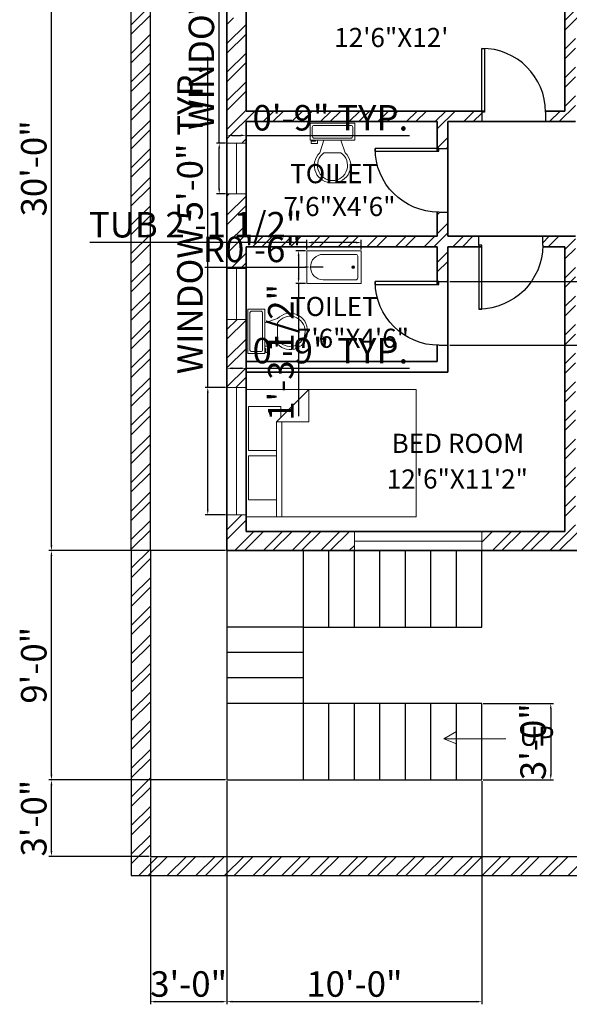
# Model space of a CAD drawing. Units: inches. Extents: x 2588 to 3237, y 2402 to 3178.
# Tile 1 of 4: x 2619 to 2878, y 2412 to 2876. Entities that reach past the tile are written whole.
import ezdxf

# ---------------------------------------------------------------- set-up
doc = ezdxf.new("R2010")
doc.units = ezdxf.units.IN
for name, color, linetype, lineweight in [('A-ANNO-DIMS', 2, 'Continuous', 18), ('A-ANNO-SYMB', 7, 'Continuous', 18), ('A-ANNO-TEXT', 7, 'Continuous', 18), ('A-AREA-IDEN', 7, 'Continuous', 25), ('A-DOOR', 3, 'Continuous', 25), ('A-FLOR-FIXT', 9, 'Continuous', 18), ('A-FLOR-STRS', 7, 'Continuous', 25), ('A-FURN', 8, 'Continuous', 18), ('A-GLAZ', 4, 'Continuous', 18), ('A-WALL-PATT', 252, 'Continuous', 13), ('L-WALL', 7, 'Continuous', 30), ('L-WALL-PATT', 252, 'Continuous', 13), ('wall', 210, 'Continuous', 35)]:
    doc.layers.add(name, color=color, linetype=linetype, lineweight=lineweight)
doc.styles.get("Standard").update_dxf_attribs({"font": 'arial.ttf'})
doc.dimstyles.new('ISO-25', dxfattribs={"dimtxt": 12, "dimasz": 2.5, "dimexe": 1.25, "dimexo": 0.625, "dimtad": 1, "dimdec": 1, "dimlunit": 4, "dimtxsty": 'Standard', "dimcen": 2.5, "dimadec": 0, "dimazin": 0, "dimtfac": 1, "dimtdec": 1, "dimtmove": 0, "dimatfit": 3, "dimfxl": 1, "dimarcsym": 0})

# ---------------------------------------------------------------- blocks, each defined once
blk = doc.blocks.new('Bed - Queen')
for p, q in [((0, -80.00003), (0, 0)), ((0, 0), (59.99999, 0)), ((59.99999, 0), (59.99999, -80.00003)), ((7.99999, -1.2), (28.79998, -1.2)), ((7.99999, -14.4), (7.99999, -1.2)), ((28.79998, -1.2), (28.79998, -14.4)), ((31.19999, -1.2), (51.99999, -1.2)), ((31.19999, -14.4), (31.19999, -1.2)), ((51.99999, -1.2), (51.99999, -16.4)), ((0, -14.4), (44.8, -14.4)), ((44.8, -16.8), (0, -16.8)), ((59.99999, -29.6), (44.8, -14.4)), ((44.8, -14.4), (44.8, -29.6)), ((51.99999, -16.4), (46.79936, -16.4)), ((44.8, -29.6), (59.99999, -29.6)), ((59.99999, -80.00003), (0, -80.00003))]:
    blk.add_line(p, q)
blk = doc.blocks.new('*U9')
for p, q in [((9.5, -6), (9.5, -2)), ((-10, -8.5), (-8, -8.5)), ((-10, -9.5), (-10, -8.5)), ((-8, -8.5), (-8, -8)), ((-7, -8), (-7, -9.5)), ((-4, -8), (-6, -14)), ((4, -8), (6, -14)), ((-7, -9.5), (-10, -9.5)), ((4, -14), (-4, -14))]:
    blk.add_line(p, q)
blk.add_lwpolyline([(10.5, -8), (10.5, 0), (-10.5, 0), (-10.5, -8)], close=True)
for points in [[(-9.5, -2), (-9.5, -6)], [(8.5, -1), (-8.5, -1)], [(-8.5, -7), (8.5, -7)]]:
    blk.add_lwpolyline(points)
for centre, radius, start, end in [((-8.625, -1.875), 0.8839, 81.8699, 188.1301), ((8.625, -1.875), 0.8839, 351.8699, 98.1301), ((-8.625, -6.125), 0.8839, 171.869898, 278.1301), ((8.625, -6.125), 0.8839, 261.8699, 8.1301), ((-0.4772, -19.9188), 8.0953, 133.01722, 273.38), ((0.0374, -19.8731), 7.127, 124.50543, 269.7), ((-0.0373, -19.8731), 7.127, 270.3, 55.4946), ((0.4773, -19.9188), 8.0953, 266.62, 46.9828)]:
    blk.add_arc(centre, radius, start, end)
blk = doc.blocks.new('Bath Tub - 26 x 60 in.')
for p, q in [((8, -18), (10, -18)), ((9, -17), (9, -19))]:
    blk.add_line(p, q)
blk.add_lwpolyline([(0, -36), (0, 0), (60, 0), (60, -36)], close=True)
for points in [[(4, -30), (4, -6)], [(6, -4), (42, -4)], [(42, -32), (6, -32)]]:
    blk.add_lwpolyline(points)
for radius in [1.5, 1]:
    blk.add_circle((9, -18), radius)
for centre, radius, start, end in [((5.75, -5.75), 1.77, 81.8699, 188.1301), ((42, -18), 14, 270, 90), ((5.75, -30.25), 1.77, 171.8699, 278.1301)]:
    blk.add_arc(centre, radius, start, end)
blk = doc.blocks.new('*U14')
for p, q in [((0, 0), (0, -6)), ((40, 0), (40, -6))]:
    blk.add_line(p, q)
blk.add_lwpolyline([(0, 0), (0, 40), (1.75, 40), (1.75, 0)], close=True)
blk.add_arc((0, 0), 40, 0, 90)
blk = doc.blocks.new('WIN-60IN')
blk.add_line((4.5, 60), (4.5, 0))
blk.add_lwpolyline([(9, 60), (9, 0), (0, 0), (0, 60)], close=True)
blk = doc.blocks.new('WIN-24IN')
blk.add_line((4.5, 0), (4.5, 24))
blk.add_lwpolyline([(0, 0), (0, 24), (9, 24), (9, 0)], close=True)
blk = doc.blocks.new('*D26')
at = {"layer": 'A-ANNO-DIMS', "color": 0, "lineweight": -2, "transparency": 16777216}
for p, q in [((2707.4, 2702.67), (2707.4, 2858.27)), ((2715.77, 2702.67), (2706.15, 2702.67)), ((2707.4, 2645.17), (2707.4, 2700.17)), ((2715.77, 2642.67), (2706.15, 2642.67))]:
    blk.add_line(p, q, dxfattribs=at)
at = {"layer": 'A-ANNO-DIMS', "color": 0, "transparency": 16777216}
for points in [[(2706.98, 2700.17), (2707.81, 2700.17), (2707.4, 2702.67)], [(2706.98, 2645.17), (2707.81, 2645.17), (2707.4, 2642.67)]]:
    blk.add_solid(points, dxfattribs=at)
at = {"layer": 'Defpoints', "color": 0, "transparency": 16777216}
for p in [(2707.4, 2702.67), (2716.4, 2702.67), (2716.4, 2642.67)]:
    blk.add_point(p, dxfattribs=at)
at = {"layer": 'A-ANNO-DIMS', "color": 0, "transparency": 16777216, "insert": (2700.56, 2781.72), "char_height": 12, "attachment_point": 5, "rotation": 90}
blk.add_mtext('WINDOW 5\'-0" TYP.', dxfattribs=at)
blk = doc.blocks.new('*D27')
at = {"layer": 'A-ANNO-DIMS', "color": 0, "lineweight": -2, "transparency": 16777216}
for p, q in [((2716.4, 2703.3), (2716.4, 2712.92)), ((2725.4, 2703.3), (2725.4, 2712.92)), ((2718.9, 2711.67), (2722.9, 2711.67)), ((2725.4, 2711.67), (2802.29, 2711.67))]:
    blk.add_line(p, q, dxfattribs=at)
at = {"layer": 'A-ANNO-DIMS', "color": 0, "transparency": 16777216}
for points in [[(2718.9, 2712.09), (2718.9, 2711.25), (2716.4, 2711.67)], [(2722.9, 2712.09), (2722.9, 2711.25), (2725.4, 2711.67)]]:
    blk.add_solid(points, dxfattribs=at)
at = {"layer": 'Defpoints', "color": 0, "transparency": 16777216}
for p in [(2725.4, 2711.67), (2716.4, 2702.67), (2725.4, 2702.67)]:
    blk.add_point(p, dxfattribs=at)
at = {"layer": 'A-ANNO-DIMS', "color": 0, "transparency": 16777216, "insert": (2765.1, 2718.42), "char_height": 12, "attachment_point": 5}
blk.add_mtext('0\'-9" TYP.', dxfattribs=at)
blk = doc.blocks.new('*D29')
at = {"layer": 'A-ANNO-DIMS', "color": 0, "lineweight": -2, "transparency": 16777216}
for p, q in [((2761.13, 2894.89), (2761.13, 2882.27)), ((2821.13, 2894.89), (2821.13, 2882.27)), ((2763.63, 2883.52), (2818.63, 2883.52)), ((2821.13, 2883.52), (2898.03, 2883.52))]:
    blk.add_line(p, q, dxfattribs=at)
at = {"layer": 'A-ANNO-DIMS', "color": 0, "transparency": 16777216}
for points in [[(2763.63, 2883.93), (2763.63, 2883.1), (2761.13, 2883.52)], [(2818.63, 2883.93), (2818.63, 2883.1), (2821.13, 2883.52)]]:
    blk.add_solid(points, dxfattribs=at)
at = {"layer": 'Defpoints', "color": 0, "transparency": 16777216}
for p in [(2761.13, 2895.52), (2821.13, 2895.52), (2821.13, 2883.52)]:
    blk.add_point(p, dxfattribs=at)
at = {"layer": 'A-ANNO-DIMS', "color": 0, "transparency": 16777216, "insert": (2860.83, 2890.27), "char_height": 12, "attachment_point": 5}
blk.add_mtext('5\'-0" TYP.', dxfattribs=at)
blk = doc.blocks.new('*D32')
at = {"layer": 'A-ANNO-DIMS', "color": 0, "lineweight": -2, "transparency": 16777216}
for p, q in [((2712.8, 2817.75), (2712.8, 2973.35)), ((2715.77, 2817.75), (2711.55, 2817.75)), ((2712.8, 2796.25), (2712.8, 2815.25)), ((2715.77, 2793.75), (2711.55, 2793.75))]:
    blk.add_line(p, q, dxfattribs=at)
at = {"layer": 'A-ANNO-DIMS', "color": 0, "transparency": 16777216}
for points in [[(2712.38, 2815.25), (2713.21, 2815.25), (2712.8, 2817.75)], [(2712.38, 2796.25), (2713.21, 2796.25), (2712.8, 2793.75)]]:
    blk.add_solid(points, dxfattribs=at)
at = {"layer": 'Defpoints', "color": 0, "transparency": 16777216}
for p in [(2712.8, 2817.75), (2716.4, 2817.75), (2716.4, 2793.75)]:
    blk.add_point(p, dxfattribs=at)
at = {"layer": 'A-ANNO-DIMS', "color": 0, "transparency": 16777216, "insert": (2705.96, 2896.8), "char_height": 12, "attachment_point": 5, "rotation": 90}
blk.add_mtext('WINDOW 2\'-0" TYP.', dxfattribs=at)
blk = doc.blocks.new('*D33')
at = {"layer": 'A-ANNO-DIMS', "color": 0, "lineweight": -2, "transparency": 16777216}
for p, q in [((2716.4, 2818.37), (2716.4, 2822.6)), ((2718.9, 2821.35), (2722.9, 2821.35)), ((2725.4, 2818.37), (2725.4, 2822.6)), ((2725.4, 2821.35), (2802.29, 2821.35))]:
    blk.add_line(p, q, dxfattribs=at)
at = {"layer": 'A-ANNO-DIMS', "color": 0, "transparency": 16777216}
for points in [[(2718.9, 2821.77), (2718.9, 2820.93), (2716.4, 2821.35)], [(2722.9, 2821.77), (2722.9, 2820.93), (2725.4, 2821.35)]]:
    blk.add_solid(points, dxfattribs=at)
at = {"layer": 'Defpoints', "color": 0, "transparency": 16777216}
for p in [(2725.4, 2821.35), (2716.4, 2817.75), (2725.4, 2817.75)]:
    blk.add_point(p, dxfattribs=at)
at = {"layer": 'A-ANNO-DIMS', "color": 0, "transparency": 16777216, "insert": (2765.1, 2828.1), "char_height": 12, "attachment_point": 5}
blk.add_mtext('0\'-9" TYP.', dxfattribs=at)
blk = doc.blocks.new('*D40')
at = {"layer": 'A-ANNO-DIMS', "color": 0, "lineweight": -2, "transparency": 16777216}
for p, q in [((2754, 2770.89), (2651.9, 2770.89)), ((2754, 2767.67), (2754, 2772.14)), ((2777.15, 2770.89), (2756.5, 2770.89)), ((2779.65, 2767.67), (2779.65, 2772.14))]:
    blk.add_line(p, q, dxfattribs=at)
at = {"layer": 'A-ANNO-DIMS', "color": 0, "transparency": 16777216}
for points in [[(2756.5, 2771.31), (2756.5, 2770.47), (2754, 2770.89)], [(2777.15, 2771.31), (2777.15, 2770.47), (2779.65, 2770.89)]]:
    blk.add_solid(points, dxfattribs=at)
at = {"layer": 'Defpoints', "color": 0, "transparency": 16777216}
for p in [(2754, 2770.89), (2754, 2767.04), (2779.65, 2767.04)]:
    blk.add_point(p, dxfattribs=at)
at = {"layer": 'A-ANNO-DIMS', "color": 0, "transparency": 16777216, "insert": (2701.7, 2777.72), "char_height": 12, "attachment_point": 5}
blk.add_mtext('TUB 2\'-1 1/2"', dxfattribs=at)
blk = doc.blocks.new('*D41')
at = {"layer": 'A-ANNO-DIMS', "color": 0, "lineweight": -2, "transparency": 16777216}
for p, q in [((2753.37, 2767.04), (2748.9, 2767.04)), ((2750.15, 2764.54), (2750.15, 2754.15)), ((2753.37, 2751.65), (2748.9, 2751.65)), ((2750.15, 2751.65), (2750.15, 2689.17))]:
    blk.add_line(p, q, dxfattribs=at)
at = {"layer": 'A-ANNO-DIMS', "color": 0, "transparency": 16777216}
for points in [[(2749.73, 2764.54), (2750.56, 2764.54), (2750.15, 2767.04)], [(2749.73, 2754.15), (2750.56, 2754.15), (2750.15, 2751.65)]]:
    blk.add_solid(points, dxfattribs=at)
at = {"layer": 'Defpoints', "color": 0, "transparency": 16777216}
for p in [(2754, 2767.04), (2750.15, 2751.65), (2754, 2751.65)]:
    blk.add_point(p, dxfattribs=at)
at = {"layer": 'A-ANNO-DIMS', "color": 0, "transparency": 16777216, "insert": (2743.31, 2719.16), "char_height": 12, "attachment_point": 5, "rotation": 90}
blk.add_mtext('1\'-3 1/2"', dxfattribs=at)
blk = doc.blocks.new('*D48')
at = {"layer": 'A-ANNO-DIMS', "color": 0, "lineweight": -2, "transparency": 16777216}
for p, q in [((2716.4, 2517.21), (2716.4, 2412.16)), ((2680.4, 2481.21), (2680.4, 2412.16)), ((2682.9, 2413.41), (2713.9, 2413.41))]:
    blk.add_line(p, q, dxfattribs=at)
at = {"layer": 'A-ANNO-DIMS', "color": 0, "transparency": 16777216}
for points in [[(2682.9, 2413.83), (2682.9, 2412.99), (2680.4, 2413.41)], [(2713.9, 2413.83), (2713.9, 2412.99), (2716.4, 2413.41)]]:
    blk.add_solid(points, dxfattribs=at)
at = {"layer": 'Defpoints', "color": 0, "transparency": 16777216}
for p in [(2716.4, 2517.83), (2680.4, 2481.83), (2716.4, 2413.41)]:
    blk.add_point(p, dxfattribs=at)
at = {"layer": 'A-ANNO-DIMS', "color": 0, "transparency": 16777216, "insert": (2698.4, 2420.17), "char_height": 12, "attachment_point": 5}
blk.add_mtext('3\'-0"', dxfattribs=at)
blk = doc.blocks.new('*D49')
at = {"layer": 'A-ANNO-DIMS', "color": 0, "lineweight": -2, "transparency": 16777216}
for p, q in [((2715.77, 2985.83), (2632.58, 2985.83)), ((2633.83, 2628.33), (2633.83, 2983.33)), ((2715.77, 2625.83), (2632.58, 2625.83))]:
    blk.add_line(p, q, dxfattribs=at)
at = {"layer": 'A-ANNO-DIMS', "color": 0, "transparency": 16777216}
for points in [[(2633.42, 2983.33), (2634.25, 2983.33), (2633.83, 2985.83)], [(2633.42, 2628.33), (2634.25, 2628.33), (2633.83, 2625.83)]]:
    blk.add_solid(points, dxfattribs=at)
at = {"layer": 'Defpoints', "color": 0, "transparency": 16777216}
for p in [(2633.83, 2985.83), (2716.4, 2985.83), (2716.4, 2625.83)]:
    blk.add_point(p, dxfattribs=at)
at = {"layer": 'A-ANNO-DIMS', "color": 0, "transparency": 16777216, "insert": (2627.08, 2805.83), "char_height": 12, "attachment_point": 5, "rotation": 90}
blk.add_mtext('30\'-0"', dxfattribs=at)
blk = doc.blocks.new('*D51')
at = {"layer": 'A-ANNO-DIMS', "color": 0, "lineweight": -2, "transparency": 16777216}
for p, q in [((2715.77, 2517.83), (2632.58, 2517.83)), ((2633.83, 2484.33), (2633.83, 2515.33)), ((2679.77, 2481.83), (2632.58, 2481.83))]:
    blk.add_line(p, q, dxfattribs=at)
at = {"layer": 'A-ANNO-DIMS', "color": 0, "transparency": 16777216}
for points in [[(2633.42, 2515.33), (2634.25, 2515.33), (2633.83, 2517.83)], [(2633.42, 2484.33), (2634.25, 2484.33), (2633.83, 2481.83)]]:
    blk.add_solid(points, dxfattribs=at)
at = {"layer": 'Defpoints', "color": 0, "transparency": 16777216}
for p in [(2633.83, 2517.83), (2716.4, 2517.83), (2680.4, 2481.83)]:
    blk.add_point(p, dxfattribs=at)
at = {"layer": 'A-ANNO-DIMS', "color": 0, "transparency": 16777216, "insert": (2627.08, 2499.83), "char_height": 12, "attachment_point": 5, "rotation": 90}
blk.add_mtext('3\'-0"', dxfattribs=at)
blk = doc.blocks.new('*D52')
at = {"layer": 'A-ANNO-DIMS', "color": 0, "lineweight": -2, "transparency": 16777216}
for p, q in [((2715.77, 2625.83), (2632.58, 2625.83)), ((2633.83, 2520.33), (2633.83, 2623.33)), ((2715.77, 2517.83), (2632.58, 2517.83))]:
    blk.add_line(p, q, dxfattribs=at)
at = {"layer": 'A-ANNO-DIMS', "color": 0, "transparency": 16777216}
for points in [[(2633.42, 2623.33), (2634.25, 2623.33), (2633.83, 2625.83)], [(2633.42, 2520.33), (2634.25, 2520.33), (2633.83, 2517.83)]]:
    blk.add_solid(points, dxfattribs=at)
at = {"layer": 'Defpoints', "color": 0, "transparency": 16777216}
for p in [(2633.83, 2625.83), (2716.4, 2625.83), (2716.4, 2517.83)]:
    blk.add_point(p, dxfattribs=at)
at = {"layer": 'A-ANNO-DIMS', "color": 0, "transparency": 16777216, "insert": (2627.08, 2571.83), "char_height": 12, "attachment_point": 5, "rotation": 90}
blk.add_mtext('9\'-0"', dxfattribs=at)
blk = doc.blocks.new('*D55')
at = {"layer": 'A-ANNO-DIMS', "color": 0, "lineweight": -2, "transparency": 16777216}
for p, q in [((2716.4, 2517.21), (2716.4, 2412.16)), ((2836.4, 2517.21), (2836.4, 2412.16)), ((2718.9, 2413.41), (2833.9, 2413.41))]:
    blk.add_line(p, q, dxfattribs=at)
at = {"layer": 'A-ANNO-DIMS', "color": 0, "transparency": 16777216}
for points in [[(2718.9, 2413.83), (2718.9, 2412.99), (2716.4, 2413.41)], [(2833.9, 2413.83), (2833.9, 2412.99), (2836.4, 2413.41)]]:
    blk.add_solid(points, dxfattribs=at)
at = {"layer": 'Defpoints', "color": 0, "transparency": 16777216}
for p in [(2716.4, 2517.83), (2836.4, 2517.83), (2836.4, 2413.41)]:
    blk.add_point(p, dxfattribs=at)
at = {"layer": 'A-ANNO-DIMS', "color": 0, "transparency": 16777216, "insert": (2776.4, 2420.16), "char_height": 12, "attachment_point": 5}
blk.add_mtext('10\'-0"', dxfattribs=at)
blk = doc.blocks.new('*D56')
at = {"layer": 'A-ANNO-DIMS', "color": 0, "lineweight": -2, "transparency": 16777216}
for p, q in [((2821.33, 2752.5), (3095.05, 2752.5)), ((3093.8, 2750), (3093.8, 2725)), ((2821.33, 2722.5), (3095.05, 2722.5)), ((3093.8, 2722.5), (3093.8, 2686.65))]:
    blk.add_line(p, q, dxfattribs=at)
at = {"layer": 'A-ANNO-DIMS', "color": 0, "transparency": 16777216}
for points in [[(3093.38, 2750), (3094.21, 2750), (3093.8, 2752.5)], [(3093.38, 2725), (3094.21, 2725), (3093.8, 2722.5)]]:
    blk.add_solid(points, dxfattribs=at)
at = {"layer": 'Defpoints', "color": 0, "transparency": 16777216}
for p in [(2820.7, 2752.5), (2820.7, 2722.5), (3093.8, 2722.5)]:
    blk.add_point(p, dxfattribs=at)
at = {"layer": 'A-ANNO-DIMS', "color": 0, "transparency": 16777216, "insert": (3087.05, 2703.33), "char_height": 12, "attachment_point": 5, "rotation": 90}
blk.add_mtext('2\'-6"', dxfattribs=at)
blk = doc.blocks.new('*D58')
at = {"layer": 'A-ANNO-DIMS', "color": 0, "lineweight": -2, "transparency": 16777216}
for p, q in [((2837.02, 2553.83), (2870.05, 2553.83)), ((2868.8, 2551.33), (2868.8, 2520.33)), ((2837.02, 2517.83), (2870.05, 2517.83))]:
    blk.add_line(p, q, dxfattribs=at)
at = {"layer": 'A-ANNO-DIMS', "color": 0, "transparency": 16777216}
for points in [[(2868.38, 2551.33), (2869.21, 2551.33), (2868.8, 2553.83)], [(2868.38, 2520.33), (2869.21, 2520.33), (2868.8, 2517.83)]]:
    blk.add_solid(points, dxfattribs=at)
at = {"layer": 'Defpoints', "color": 0, "transparency": 16777216}
for p in [(2836.4, 2553.83), (2836.4, 2517.83), (2868.8, 2517.83)]:
    blk.add_point(p, dxfattribs=at)
at = {"layer": 'A-ANNO-DIMS', "color": 0, "transparency": 16777216, "insert": (2862.04, 2535.83), "char_height": 12, "attachment_point": 5, "rotation": 90}
blk.add_mtext('3\'-0"', dxfattribs=at)
blk = doc.blocks.new('*D64')
at = {"layer": 'A-ANNO-DIMS', "color": 0, "lineweight": -2, "transparency": 16777216}
for p, q in [((2706.07, 2759.35), (2753.21, 2759.35)), ((2761.69, 2759.34), (2755.71, 2759.35))]:
    blk.add_line(p, q, dxfattribs=at)
at = {"layer": 'A-ANNO-DIMS', "color": 0, "transparency": 16777216}
blk.add_solid([(2753.21, 2759.76), (2753.21, 2758.93), (2755.71, 2759.35)], dxfattribs=at)
at = {"layer": 'Defpoints', "color": 0, "transparency": 16777216}
for p in [(2755.71, 2759.35), (2761.69, 2759.34)]:
    blk.add_point(p, dxfattribs=at)
at = {"layer": 'A-ANNO-DIMS', "color": 0, "transparency": 16777216, "insert": (2728.39, 2766.1), "char_height": 12, "attachment_point": 5, "rotation": 359.9989}
blk.add_mtext('R0\'-6"', dxfattribs=at)

msp = doc.modelspace()

# ---------------------------------------------------------------- hatches: boundary and pattern name
at = {"layer": 'A-WALL-PATT'}
h = msp.add_hatch(dxfattribs=at)
h.set_pattern_fill('ANSI32', color=256)
h.paths.add_polyline_path([(3016.4, 2985.83), (2995.46, 2985.83), (2995.46, 2976.83), (3007.4, 2976.83), (3007.4, 2880.83), (2973.06, 2880.83), (2973.06, 2875.83), (3007.4, 2875.83), (3007.4, 2760.26), (3016.4, 2760.26)])
h.paths.add_polyline_path([(2899.05, 2630.33, -0.03766), (2899.39, 2634.83), (2880.4, 2634.83), (2880.4, 2773.83), (2865, 2773.83), (2865, 2769.59, -0.00634), (2864.99, 2768.83), (2875.4, 2768.83), (2875.4, 2634.83), (2836.4, 2634.83), (2836.4, 2625.83), (2899.05, 2625.83)])
h.paths.add_polyline_path([(2725.4, 2734.72), (2716.4, 2734.72), (2716.4, 2702.67), (2725.4, 2702.67)])
h.paths.add_polyline_path([(2776.4, 2634.83), (2725.4, 2634.83), (2725.4, 2642.67), (2716.4, 2642.67), (2716.4, 2625.83), (2776.4, 2625.83)])
h.paths.add_polyline_path([(2725.4, 2793.75), (2716.4, 2793.75), (2716.4, 2758.72), (2725.4, 2758.72), (2725.4, 2768.83), (2815.4, 2768.83), (2815.4, 2752.5), (2816.2, 2752.5), (2820.4, 2752.5), (2820.4, 2768.83), (2835, 2768.83), (2835, 2769.59), (2835, 2773.83), (2820.4, 2773.83), (2820.4, 2785.18), (2816.11, 2785.18, -0.005966), (2815.4, 2785.19), (2815.4, 2773.83), (2725.4, 2773.83)])
h.paths.add_polyline_path([(2725.4, 2876.72), (2716.4, 2876.72), (2716.4, 2817.75), (2725.4, 2817.75), (2725.4, 2827.83), (2815.4, 2827.83), (2815.4, 2815.18), (2816.11, 2815.18), (2820.4, 2815.18), (2820.4, 2827.83), (2836.34, 2827.83), (2836.34, 2832.33), (2836.34, 2832.83), (2725.4, 2832.83)])
h.paths.add_polyline_path([(2725.4, 2976.83), (2764.42, 2976.83), (2764.42, 2985.83), (2716.4, 2985.83), (2716.4, 2936.72), (2725.4, 2936.72)])
h.paths.add_polyline_path([(2935.46, 2985.83), (2824.42, 2985.83), (2824.42, 2976.83), (2875.4, 2976.83), (2875.4, 2832.83), (2866.34, 2832.83, -0.004167), (2866.34, 2832.33), (2866.34, 2827.83), (2880.4, 2827.83), (2880.4, 2875.83), (2906.11, 2875.83), (2906.11, 2880.83), (2880.4, 2880.83), (2880.4, 2976.83), (2935.46, 2976.83)])
at = {"layer": 'L-WALL-PATT'}
h = msp.add_hatch(dxfattribs=at)
h.set_pattern_fill('ANSI32', color=256)
h.paths.add_polyline_path([(3016.4, 2700.26), (3007.4, 2700.26), (3007.4, 2634.83), (2956.08, 2634.83, -0.03766), (2956.42, 2630.33), (2956.42, 2625.83), (3016.4, 2625.83)], flags=17)
h.paths.add_polyline_path([(3061.4, 2985.83), (3061.4, 3021.83), (3061.4, 3030.83), (3052.4, 3030.83), (3016.4, 3030.83), (2716.4, 3030.83), (2680.4, 3030.83), (2671.4, 3030.83), (2671.4, 3021.83), (2671.4, 2985.83), (2671.4, 2625.83), (2671.4, 2481.83), (2671.4, 2472.83), (2680.4, 2472.83), (2716.4, 2472.83), (2836.4, 2472.83), (2900.91, 2472.83), (2900.91, 2481.83), (2836.4, 2481.83), (2716.4, 2481.83), (2680.4, 2481.83), (2680.4, 2625.83), (2680.4, 2985.83), (2680.4, 3021.83), (2716.4, 3021.83), (3016.4, 3021.83), (3052.4, 3021.83), (3052.4, 2985.83), (3052.4, 2625.83), (3052.4, 2481.83), (2984.91, 2481.83), (2984.91, 2472.83), (3052.4, 2472.83), (3061.4, 2472.83), (3061.4, 2481.83), (3061.4, 2625.83)])

# ---------------------------------------------------------------- linework, layer by layer
at = {"layer": 'A-ANNO-SYMB'}
for p, q in [((2818.47, 2537.2), (2824.4, 2540.66)), ((2847.69, 2537.2), (2818.47, 2537.2)), ((2818.47, 2537.2), (2824.4, 2534.87))]:
    msp.add_line(p, q, dxfattribs=at)
at = {"layer": 'A-FLOR-STRS'}
for p, q in [((2716.4, 2625.83), (2716.4, 2517.83)), ((2752.4, 2589.83), (2752.4, 2625.83)), ((2764.4, 2589.83), (2764.4, 2625.83)), ((2776.4, 2589.83), (2776.4, 2625.83)), ((2788.4, 2589.83), (2788.4, 2625.83)), ((2800.4, 2589.83), (2800.4, 2625.83)), ((2812.4, 2589.83), (2812.4, 2625.83)), ((2824.4, 2589.83), (2824.4, 2625.83)), ((2836.4, 2589.83), (2836.4, 2625.83)), ((2752.4, 2589.83), (2716.4, 2589.83)), ((2752.4, 2553.83), (2752.4, 2589.83)), ((2752.4, 2589.83), (2836.4, 2589.83)), ((2752.4, 2577.83), (2716.4, 2577.83)), ((2752.4, 2565.83), (2716.4, 2565.83)), ((2752.4, 2553.83), (2716.4, 2553.83)), ((2836.4, 2553.83), (2752.4, 2553.83)), ((2752.4, 2517.83), (2752.4, 2553.83)), ((2764.4, 2517.83), (2764.4, 2553.83)), ((2776.4, 2517.83), (2776.4, 2553.83)), ((2788.4, 2517.83), (2788.4, 2553.83)), ((2800.4, 2517.83), (2800.4, 2553.83)), ((2812.4, 2517.83), (2812.4, 2553.83)), ((2824.4, 2517.83), (2824.4, 2553.83)), ((2836.4, 2517.83), (2836.4, 2553.83)), ((2716.4, 2517.83), (2836.4, 2517.83))]:
    msp.add_line(p, q, dxfattribs=at)
at = {"layer": 'L-WALL'}
for p, q in [((2671.4, 2625.83), (2671.4, 2985.83)), ((2680.4, 2625.83), (2680.4, 2985.83)), ((2671.4, 2625.83), (2671.4, 2481.83)), ((2680.4, 2625.83), (2680.4, 2481.83)), ((2671.4, 2481.83), (2671.4, 2472.83)), ((2680.4, 2481.83), (2716.4, 2481.83)), ((2716.4, 2481.83), (2836.4, 2481.83)), ((2836.4, 2481.83), (3052.4, 2481.83)), ((2671.4, 2472.83), (2680.4, 2472.83)), ((2680.4, 2472.83), (2716.4, 2472.83)), ((2716.4, 2472.83), (2836.4, 2472.83)), ((2836.4, 2472.83), (3052.4, 2472.83))]:
    msp.add_line(p, q, dxfattribs=at)
at = {"layer": 'wall'}
for p, q in [((2716.4, 2625.83), (2716.4, 2985.83)), ((2725.4, 2832.83), (2725.4, 2976.83)), ((2875.4, 2832.83), (2875.4, 2976.83)), ((2725.4, 2832.83), (2837.66, 2832.83)), ((2866.34, 2832.83), (2875.4, 2832.83)), ((2725.4, 2827.83), (2815.4, 2827.83)), ((2725.4, 2773.83), (2725.4, 2827.83)), ((2815.4, 2813.86), (2815.4, 2827.83)), ((2820.4, 2773.83), (2820.4, 2827.83)), ((2820.4, 2827.83), (2880.4, 2827.83)), ((2815.4, 2773.83), (2815.4, 2785.19)), ((2725.4, 2773.83), (2815.4, 2773.83)), ((2820.4, 2773.83), (2880.4, 2773.83)), ((2725.4, 2634.83), (2725.4, 2768.83)), ((2725.4, 2768.83), (2815.4, 2768.83)), ((2815.4, 2751.19), (2815.4, 2768.83)), ((2820.4, 2709.83), (2820.4, 2768.83)), ((2820.4, 2768.83), (2836.31, 2768.83)), ((2864.99, 2768.83), (2875.4, 2768.83)), ((2875.4, 2634.83), (2875.4, 2768.83)), ((2815.4, 2714.83), (2815.4, 2722.52)), ((2725.4, 2714.83), (2815.4, 2714.83)), ((2725.4, 2709.83), (2820.4, 2709.83)), ((2875.4, 2634.83), (2725.4, 2634.83)), ((3016.4, 2625.83), (2716.4, 2625.83))]:
    msp.add_line(p, q, dxfattribs=at)

# ---------------------------------------------------------------- block references
at = {"layer": 'A-DOOR', "xscale": 0.75, "yscale": 0.75, "zscale": 0.75}
msp.add_blockref('*U14', (2836.34, 2832.33), dxfattribs=at)
at = {"layer": 'A-DOOR', "xscale": -0.75, "yscale": 0.75, "zscale": 0.75}
for p, rotation in [((2816.11, 2815.18), 90), ((2835, 2769.59), 180), ((2816.2, 2752.5), 90)]:
    msp.add_blockref('*U14', p, dxfattribs=dict(at, rotation=rotation))
at = {"layer": 'A-FLOR-FIXT'}
msp.add_blockref('*U9', (2766.09, 2827.06), dxfattribs=at)
at = {"layer": 'A-FLOR-FIXT', "xscale": 0.4276420079334761, "yscale": 0.4276420079334761, "zscale": 0.4276420079334761, "rotation": 180}
msp.add_blockref('Bath Tub - 26 x 60 in.', (2779.65, 2751.65), dxfattribs=at)
at = {"layer": 'A-FLOR-FIXT', "rotation": 90}
msp.add_blockref('*U9', (2726.23, 2729.06), dxfattribs=at)
at = {"layer": 'A-FURN', "rotation": 90}
msp.add_blockref('Bed - Queen', (2725.4, 2641.68), dxfattribs=at)
at = {"layer": 'A-GLAZ'}
for name, p in [('WIN-24IN', (2716.4, 2793.75)), ('WIN-24IN', (2716.4, 2734.72)), ('WIN-60IN', (2716.4, 2642.67))]:
    msp.add_blockref(name, p, dxfattribs=at)
at = {"layer": 'A-GLAZ', "rotation": 89.9999999999983}
msp.add_blockref('WIN-60IN', (2836.4, 2625.83), dxfattribs=at)

# ---------------------------------------------------------------- texts
at = {"layer": 'A-ANNO-TEXT'}
msp.add_text('UP', height=9, dxfattribs=at).set_placement((2854.01, 2533.89))
at = {"layer": 'A-AREA-IDEN'}
for s, p in [('12\'6"X12\'', (2766.89, 2862.96)), ('TOILET', (2746.17, 2798.83)), ('7\'6"X4\'6"', (2742.99, 2783.37)), ('TOILET', (2746.11, 2736.3)), ('7\'6"X4\'6"', (2749.34, 2721.3)), ('BED ROOM', (2793.89, 2671.83)), ('12\'6"X11\'2"', (2791.66, 2655.03))]:
    msp.add_text(s, height=9, dxfattribs=at).set_placement(p)

# ---------------------------------------------------------------- dimensions: what is measured, and where the dimension line sits
at = {"layer": 'A-ANNO-DIMS'}
for base, p1, p2, angle, picture, middle in [((2633.83, 2985.83), (2716.4, 2625.83), (2716.4, 2985.83), 90, '*D49', (2627.08, 2805.83)), ((2750.15, 2751.65), (2754, 2767.04), (2754, 2751.65), 270, '*D41', (2743.31, 2719.16)), ((3093.8, 2722.5), (2820.7, 2752.5), (2820.7, 2722.5), 90, '*D56', (3087.05, 2703.33)), ((2633.83, 2625.83), (2716.4, 2517.83), (2716.4, 2625.83), 90, '*D52', (2627.08, 2571.83)), ((2868.8, 2517.83), (2836.4, 2553.83), (2836.4, 2517.83), 270, '*D58', (2862.04, 2535.83)), ((2633.83, 2517.83), (2680.4, 2481.83), (2716.4, 2517.83), 90, '*D51', (2627.08, 2499.83))]:
    dim = msp.add_linear_dim(base=base, p1=p1, p2=p2, angle=angle, dimstyle='ISO-25', override={"dimdec": 1, "dimlfac": 1, "dimrnd": 0, "dimzin": 1, "dimdsep": 46, "dimlunit": 4, "dimfrac": 2}, dxfattribs=at)
    dim.commit()
    dim.dimension.update_dxf_attribs({"geometry": picture, "text_midpoint": middle})
for base, p1, p2, angle, text, picture, middle in [((2712.8, 2817.75), (2716.4, 2793.75), (2716.4, 2817.75), 90, 'WINDOW <> TYP.', '*D32', (2705.96, 2896.8)), ((2707.4, 2702.67), (2716.4, 2642.67), (2716.4, 2702.67), 90, 'WINDOW <> TYP.', '*D26', (2700.56, 2781.72)), ((2753.9959, 2770.8912), (2779.6544, 2767.0424), (2753.9959, 2767.0424), 180, 'TUB <>', '*D40', (2701.6963, 2777.7209))]:
    dim = msp.add_linear_dim(base=base, p1=p1, p2=p2, angle=angle, text=text, dimstyle='ISO-25', override={"dimdec": 1, "dimlfac": 1, "dimrnd": 0, "dimzin": 1, "dimdsep": 46, "dimlunit": 4, "dimfrac": 2}, dxfattribs=at)
    dim.commit()
    dim.dimension.update_dxf_attribs({"geometry": picture, "text_midpoint": middle})
for base, p1, p2, picture, middle in [((2821.13, 2883.52), (2761.13, 2895.52), (2821.13, 2895.52), '*D29', (2860.83, 2890.27)), ((2725.4, 2821.35), (2716.4, 2817.75), (2725.4, 2817.75), '*D33', (2765.1, 2828.1)), ((2725.4, 2711.67), (2716.4, 2702.67), (2725.4, 2702.67), '*D27', (2765.1, 2718.42))]:
    dim = msp.add_linear_dim(base=base, p1=p1, p2=p2, text='<> TYP.', dimstyle='ISO-25', override={"dimdec": 1, "dimlfac": 1, "dimrnd": 0, "dimzin": 1, "dimdsep": 46, "dimlunit": 4, "dimfrac": 2}, dxfattribs=at)
    dim.commit()
    dim.dimension.update_dxf_attribs({"geometry": picture, "text_midpoint": middle})
dim = msp.add_radius_dim(center=(2761.69, 2759.34), mpoint=(2755.71, 2759.35), dimstyle='ISO-25', override={"dimdec": 1, "dimlfac": 1, "dimrnd": 0, "dimzin": 1, "dimdsep": 46, "dimlunit": 4, "dimfrac": 2}, dxfattribs=at)
dim.commit()
dim.dimension.update_dxf_attribs({"geometry": '*D64', "text_midpoint": (2728.39, 2766.1)})
for base, p1, p2, picture, middle in [((2716.4, 2413.41), (2680.4, 2481.83), (2716.4, 2517.83), '*D48', (2698.4, 2420.17)), ((2836.4, 2413.41), (2716.4, 2517.83), (2836.4, 2517.83), '*D55', (2776.4, 2420.16))]:
    dim = msp.add_linear_dim(base=base, p1=p1, p2=p2, dimstyle='ISO-25', override={"dimdec": 1, "dimlfac": 1, "dimrnd": 0, "dimzin": 1, "dimdsep": 46, "dimlunit": 4, "dimfrac": 2}, dxfattribs=at)
    dim.commit()
    dim.dimension.update_dxf_attribs({"geometry": picture, "text_midpoint": middle})

doc.saveas('drawing.dxf')
